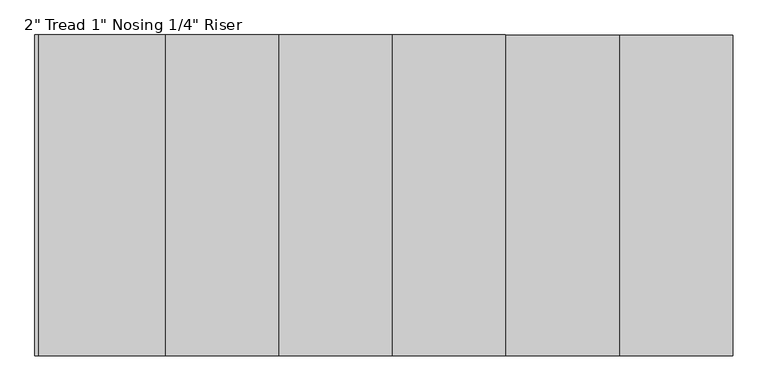
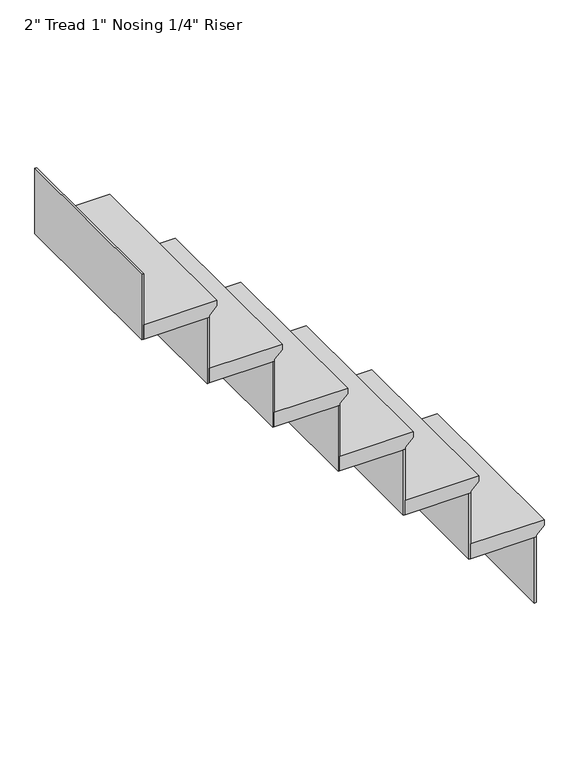
"""IFC4 building model written with IfcOpenShell, lengths in millimetres: stair flight geometry."""

from ifc_helpers import new_model, si_unit, frame, origin, place, context, project, spatial, polyline, outline, extrude, source, transform, mapped, element, save


def stair_flight_03d0a82c(model_context):
    return source(origin(), model_context, "Body", "SweptSolid", [
        extrude(outline(polyline([(1828.8, -3732.7409298), (1828.8, -3974.0409298), (1778.0, -3974.0409298), (1778.0, -3758.1409298), (1784.35, -3758.1409298), (1809.75, -3732.7409298), (1828.8, -3732.7409298)])), frame((0.0, -4554.9664375, 0.0), z_axis=(0.0, 1.0, 0.0), x_axis=(0.0, 0.0, 1.0)), (0.0, 0.0, 1.0), 609.6),
        extrude(outline(polyline([(-3764.4909298, -3945.3664375), (-3758.1409298, -3945.3664375), (-3758.1409298, -4554.9664375), (-3764.4909298, -4554.9664375), (-3764.4909298, -3945.3664375)])), frame((0.0, 0.0, 1549.4), z_axis=(0.0, 0.0, 1.0), x_axis=(1.0, 0.0, 0.0)), (0.0, 0.0, 1.0), 228.6),
        extrude(outline(polyline([(-3980.3909298, -3945.3664375), (-3974.0409298, -3945.3664375), (-3974.0409298, -4554.9664375), (-3980.3909298, -4554.9664375), (-3980.3909298, -3945.3664375)])), frame((0.0, 0.0, 1778.0), z_axis=(0.0, 0.0, 1.0), x_axis=(1.0, 0.0, 0.0)), (0.0, 0.0, 1.0), 228.6),
        extrude(outline(polyline([(2057.4, -3948.6409298), (2057.4, -4189.9409298), (2006.6, -4189.9409298), (2006.6, -3974.0409298), (2012.95, -3974.0409298), (2038.35, -3948.6409298), (2057.4, -3948.6409298)])), frame((0.0, -4554.9664375, 0.0), z_axis=(0.0, 1.0, 0.0), x_axis=(0.0, 0.0, 1.0)), (0.0, 0.0, 1.0), 609.6),
        extrude(outline(polyline([(-4196.2909298, -3945.3664375), (-4189.9409298, -3945.3664375), (-4189.9409298, -4554.9664375), (-4196.2909298, -4554.9664375), (-4196.2909298, -3945.3664375)])), frame((0.0, 0.0, 2006.6), z_axis=(0.0, 0.0, 1.0), x_axis=(1.0, 0.0, 0.0)), (0.0, 0.0, 1.0), 228.6),
        extrude(outline(polyline([(2286.0, -4164.5409298), (2286.0, -4405.8409298), (2235.2, -4405.8409298), (2235.2, -4189.9409298), (2241.55, -4189.9409298), (2266.95, -4164.5409298), (2286.0, -4164.5409298)])), frame((0.0, -4554.9664375, 0.0), z_axis=(0.0, 1.0, 0.0), x_axis=(0.0, 0.0, 1.0)), (0.0, 0.0, 1.0), 609.6),
        extrude(outline(polyline([(-4412.1909298, -3945.3664375), (-4405.8409298, -3945.3664375), (-4405.8409298, -4554.9664375), (-4412.1909298, -4554.9664375), (-4412.1909298, -3945.3664375)])), frame((0.0, 0.0, 2235.2), z_axis=(0.0, 0.0, 1.0), x_axis=(1.0, 0.0, 0.0)), (0.0, 0.0, 1.0), 228.6),
        extrude(outline(polyline([(2514.6, -4380.4409298), (2514.6, -4621.7409298), (2463.8, -4621.7409298), (2463.8, -4405.8409298), (2470.15, -4405.8409298), (2495.55, -4380.4409298), (2514.6, -4380.4409298)])), frame((0.0, -4554.9664375, 0.0), z_axis=(0.0, 1.0, 0.0), x_axis=(0.0, 0.0, 1.0)), (0.0, 0.0, 1.0), 609.6),
        extrude(outline(polyline([(-4628.0909298, -3945.3664375), (-4621.7409298, -3945.3664375), (-4621.7409298, -4554.9664375), (-4628.0909298, -4554.9664375), (-4628.0909298, -3945.3664375)])), frame((0.0, 0.0, 2463.8), z_axis=(0.0, 0.0, 1.0), x_axis=(1.0, 0.0, 0.0)), (0.0, 0.0, 1.0), 228.6),
        extrude(outline(polyline([(2743.2, -4596.3409298), (2743.2, -4837.6409298), (2692.4, -4837.6409298), (2692.4, -4621.7409298), (2698.75, -4621.7409298), (2724.15, -4596.3409298), (2743.2, -4596.3409298)])), frame((0.0, -4554.9664375, 0.0), z_axis=(0.0, 1.0, 0.0), x_axis=(0.0, 0.0, 1.0)), (0.0, 0.0, 1.0), 609.6),
        extrude(outline(polyline([(-4843.9909298, -3945.3664375), (-4837.6409298, -3945.3664375), (-4837.6409298, -4554.9664375), (-4843.9909298, -4554.9664375), (-4843.9909298, -3945.3664375)])), frame((0.0, 0.0, 2692.4), z_axis=(0.0, 0.0, 1.0), x_axis=(1.0, 0.0, 0.0)), (0.0, 0.0, 1.0), 228.6),
        extrude(outline(polyline([(-5059.8909298, -3945.3664375), (-5053.5409298, -3945.3664375), (-5053.5409298, -4554.9664375), (-5059.8909298, -4554.9664375), (-5059.8909298, -3945.3664375)])), frame((0.0, 0.0, 2921.0), z_axis=(0.0, 0.0, 1.0), x_axis=(1.0, 0.0, 0.0)), (0.0, 0.0, 1.0), 228.6),
        extrude(outline(polyline([(2971.8, -4812.2409298), (2971.8, -5053.5409298), (2921.0, -5053.5409298), (2921.0, -4837.6409298), (2927.35, -4837.6409298), (2952.75, -4812.2409298), (2971.8, -4812.2409298)])), frame((0.0, -4554.9664375, 0.0), z_axis=(0.0, 1.0, 0.0), x_axis=(0.0, 0.0, 1.0)), (0.0, 0.0, 1.0), 609.6),
    ])


if __name__ == "__main__":
    model = new_model("IFC4")
    model_context = context("Model", 3, world=origin())
    ifc_project = project(units=[si_unit("LENGTHUNIT", "METRE", prefix="MILLI")], contexts=[model_context])
    site = spatial("IfcSite", under=ifc_project)
    building = spatial("IfcBuilding", under=site)
    placement = place(None, origin())
    stair_flight_shape = stair_flight_03d0a82c(model_context)
    element("IfcStairFlight", 1, ObjectType="2\" Tread 1\" Nosing 1/4\" Riser", at=placement, inside=building, context=model_context, shape_type="MappedRepresentation", body=[
        mapped(stair_flight_shape, transform((0.0, 0.0, 0.0), x_axis=(1.0, 0.0, 0.0), y_axis=(0.0, 1.0, 0.0), z_axis=(0.0, 0.0, 1.0))),
    ])
    save(model, "model.ifc")
